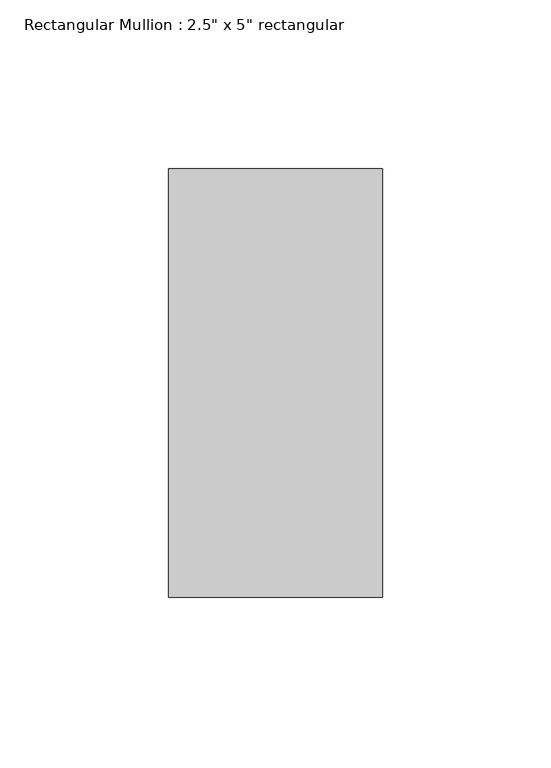
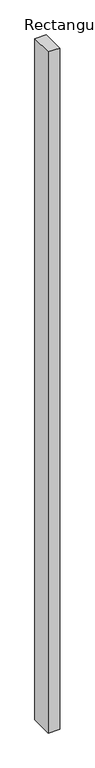
"""IFC4 building model written with IfcOpenShell, lengths in millimetres: member geometry."""

from ifc_helpers import new_model, si_unit, frame, origin, place, context, project, spatial, polyline, outline, extrude, source, transform, mapped, element, save


def member_e5c989f4(model_context):
    return source(origin(), model_context, "Body", "SweptSolid", [
        extrude(outline(polyline([(31.75, 63.5), (31.75, -63.5), (-31.75, -63.5), (-31.75, 63.5), (31.75, 63.5)])), frame((0.0, 0.0, -3962.4), z_axis=(0.0, 0.0, 1.0), x_axis=(1.0, 0.0, 0.0)), (0.0, 0.0, 1.0), 3962.4),
    ])


if __name__ == "__main__":
    model = new_model("IFC4")
    model_context = context("Model", 3, world=origin())
    ifc_project = project(units=[si_unit("LENGTHUNIT", "METRE", prefix="MILLI")], contexts=[model_context])
    site = spatial("IfcSite", under=ifc_project)
    building = spatial("IfcBuilding", under=site)
    placement = place(None, origin())
    member_shape = member_e5c989f4(model_context)
    element("IfcMember", 1, ObjectType="Rectangular Mullion : 2.5\" x 5\" rectangular", at=placement, inside=building, context=model_context, shape_type="MappedRepresentation", body=[
        mapped(member_shape, transform((0.0, 0.0, 0.0), x_axis=(1.0, 0.0, 0.0), y_axis=(0.0, 1.0, 0.0), z_axis=(0.0, 0.0, 1.0))),
    ])
    save(model, "model.ifc")

# Revit data of these elements
# Type "Rectangular Mullion : 2.5\" x 5\" rectangular"
#   built-in parameter 1007304 = 0.416667 (stored number, unit not read)
#   built-in parameter 1007301 = 0.104167 (stored number, unit not read)
#   built-in parameter 1007300 = 0.104167 (stored number, unit not read)
# Element 1 (IfcMember, "Rectangular Mullion : 2.5\" x 5\" rectangular")
#   Materials on its faces: "Iron, Ductile"
# Materials
#   "Iron, Ductile": class "Metal", colour RGB 0 0 0, transparency 0, Description = "Ductile cast iron", Cost = 0
